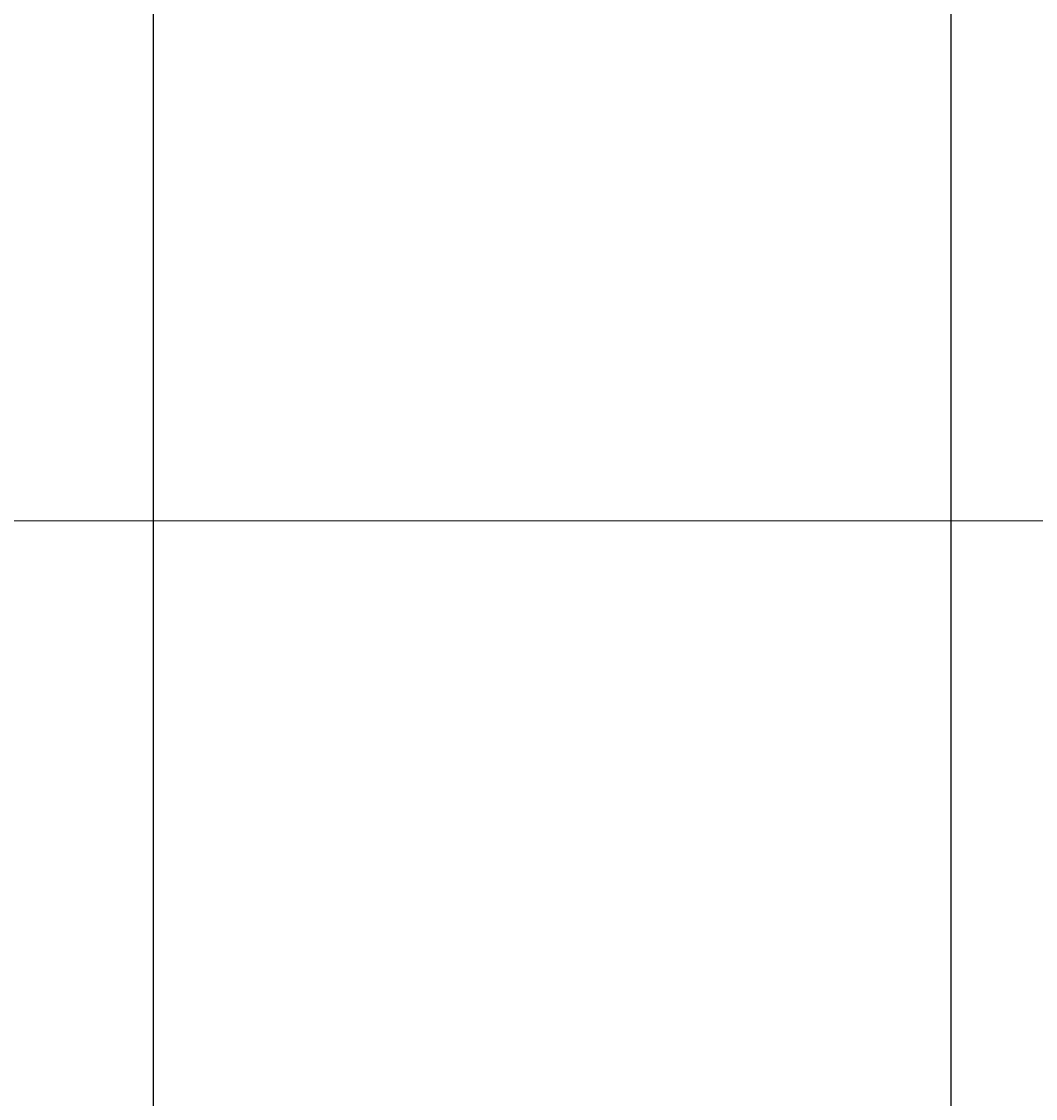
# Model space of a CAD drawing. Units: inches. Extents: x 738 to 1068, y 378 to 757.
# Tile 26 of 41: x 806 to 833, y 578 to 606. Entities that reach past the tile are written whole.
import ezdxf

# ---------------------------------------------------------------- set-up
doc = ezdxf.new("R2010")
doc.units = ezdxf.units.IN
doc.header["$MEASUREMENT"] = 0
doc.layers.add('A-ANNO-DIMS', color=2, linetype='Continuous', lineweight=18)
doc.layers.add('E-CTRL-WIRE', color=7, linetype='Continuous', lineweight=18)
doc.styles.get("Standard").update_dxf_attribs({"font": 'arial.ttf'})
doc.dimstyles.get("Standard").update_dxf_attribs({"dimtxt": 0.18, "dimasz": 0.18, "dimexe": 0.18, "dimexo": 0.0625, "dimgap": 0.09, "dimtad": 0, "dimtih": 1, "dimtoh": 1, "dimdec": 4, "dimzin": 0, "dimdsep": 46, "dimtxsty": 'Standard', "dimcen": 0.09, "dimadec": 0, "dimazin": 0, "dimtfac": 1, "dimtdec": 4, "dimtofl": 0, "dimtmove": 0, "dimatfit": 3, "dimfxl": 1, "dimtolj": 1, "dimtzin": 0, "dimarcsym": 0})

# ---------------------------------------------------------------- blocks, each defined once
blk = doc.blocks.new('*D32')
at = {"layer": 'A-ANNO-DIMS', "color": 0, "lineweight": -2, "transparency": 16777216}
for p, q in [((809.38, 461.454), (809.38, 756.505)), ((836.232, 461.277), (836.232, 756.505)), ((809.56, 756.325), (822.41, 756.325)), ((836.052, 756.325), (823.202, 756.325))]:
    blk.add_line(p, q, dxfattribs=at)
at = {"layer": 'A-ANNO-DIMS', "color": 0, "transparency": 16777216}
for points in [[(809.56, 756.355), (809.56, 756.295), (809.38, 756.325)], [(836.052, 756.355), (836.052, 756.295), (836.232, 756.325)]]:
    blk.add_solid(points, dxfattribs=at)
at = {"layer": 'Defpoints', "color": 0, "transparency": 16777216}
for p in [(836.232, 756.325), (809.38, 461.392), (836.232, 461.214)]:
    blk.add_point(p, dxfattribs=at)
at = {"layer": 'A-ANNO-DIMS', "color": 0, "transparency": 16777216, "insert": (822.806, 756.325), "char_height": 0.18, "attachment_point": 5}
blk.add_mtext('\\A1;26.85', dxfattribs=at)
blk = doc.blocks.new('*D34')
at = {"layer": 'A-ANNO-DIMS', "color": 0, "lineweight": -2, "transparency": 16777216}
for p, q in [((781.49, 686.266), (781.49, 378.239)), ((830.489, 686.266), (830.489, 378.239)), ((781.67, 378.419), (805.767, 378.419)), ((830.309, 378.419), (806.212, 378.419))]:
    blk.add_line(p, q, dxfattribs=at)
at = {"layer": 'A-ANNO-DIMS', "color": 0, "transparency": 16777216}
for points in [[(781.67, 378.449), (781.67, 378.389), (781.49, 378.419)], [(830.309, 378.449), (830.309, 378.389), (830.489, 378.419)]]:
    blk.add_solid(points, dxfattribs=at)
at = {"layer": 'Defpoints', "color": 0, "transparency": 16777216}
for p in [(781.49, 686.329), (830.489, 686.329), (830.489, 378.419)]:
    blk.add_point(p, dxfattribs=at)
at = {"layer": 'A-ANNO-DIMS', "color": 0, "transparency": 16777216, "insert": (805.99, 378.419), "char_height": 0.18, "attachment_point": 5}
blk.add_mtext('\\A1;49', dxfattribs=at)
blk = doc.blocks.new('*D38')
at = {"layer": 'A-ANNO-DIMS', "color": 0, "lineweight": -2, "transparency": 16777216}
for p, q in [((781.485, 593.017), (781.485, 378.239)), ((887.04, 593.067), (887.04, 378.239)), ((781.665, 378.419), (833.807, 378.419)), ((886.86, 378.419), (834.718, 378.419))]:
    blk.add_line(p, q, dxfattribs=at)
at = {"layer": 'A-ANNO-DIMS', "color": 0, "transparency": 16777216}
for points in [[(781.665, 378.449), (781.665, 378.389), (781.485, 378.419)], [(886.86, 378.449), (886.86, 378.389), (887.04, 378.419)]]:
    blk.add_solid(points, dxfattribs=at)
at = {"layer": 'Defpoints', "color": 0, "transparency": 16777216}
for p in [(781.485, 593.08), (887.04, 593.13), (887.04, 378.419)]:
    blk.add_point(p, dxfattribs=at)
at = {"layer": 'A-ANNO-DIMS', "color": 0, "transparency": 16777216, "insert": (834.263, 378.419), "char_height": 0.18, "attachment_point": 5}
blk.add_mtext('\\A1;105.56', dxfattribs=at)

msp = doc.modelspace()

# ---------------------------------------------------------------- linework, layer by layer
at = {"layer": 'E-CTRL-WIRE'}
msp.add_line((781.4897, 593.1296), (887.0404, 593.1296), dxfattribs=at)

# ---------------------------------------------------------------- dimensions: what is measured, and where the dimension line sits
at = {"layer": 'A-ANNO-DIMS'}
for base, p1, p2, override, picture, middle in [((836.2324, 756.3251), (809.3803, 461.3919), (836.2324, 461.214), {"dimdec": 2, "dimlfac": 1, "dimrnd": 0, "dimzin": 0, "dimdsep": 46, "dimlunit": 2}, '*D32', (822.8064, 756.3251)), ((830.4893, 378.4191), (781.4897, 686.329), (830.4893, 686.329), {"dimdec": 0, "dimlfac": 1, "dimrnd": 0, "dimzin": 0, "dimdsep": 46, "dimlunit": 2}, '*D34', (805.9895, 378.4191)), ((887.0404, 378.4191), (781.4846, 593.0796), (887.0404, 593.1296), {"dimdec": 2, "dimlfac": 1, "dimrnd": 0, "dimzin": 0, "dimdsep": 46, "dimlunit": 2}, '*D38', (834.2625, 378.4191))]:
    dim = msp.add_linear_dim(base=base, p1=p1, p2=p2, dimstyle='Standard', override=override, dxfattribs=at)
    dim.commit()
    dim.dimension.update_dxf_attribs({"geometry": picture, "text_midpoint": middle})

doc.saveas('drawing.dxf')
